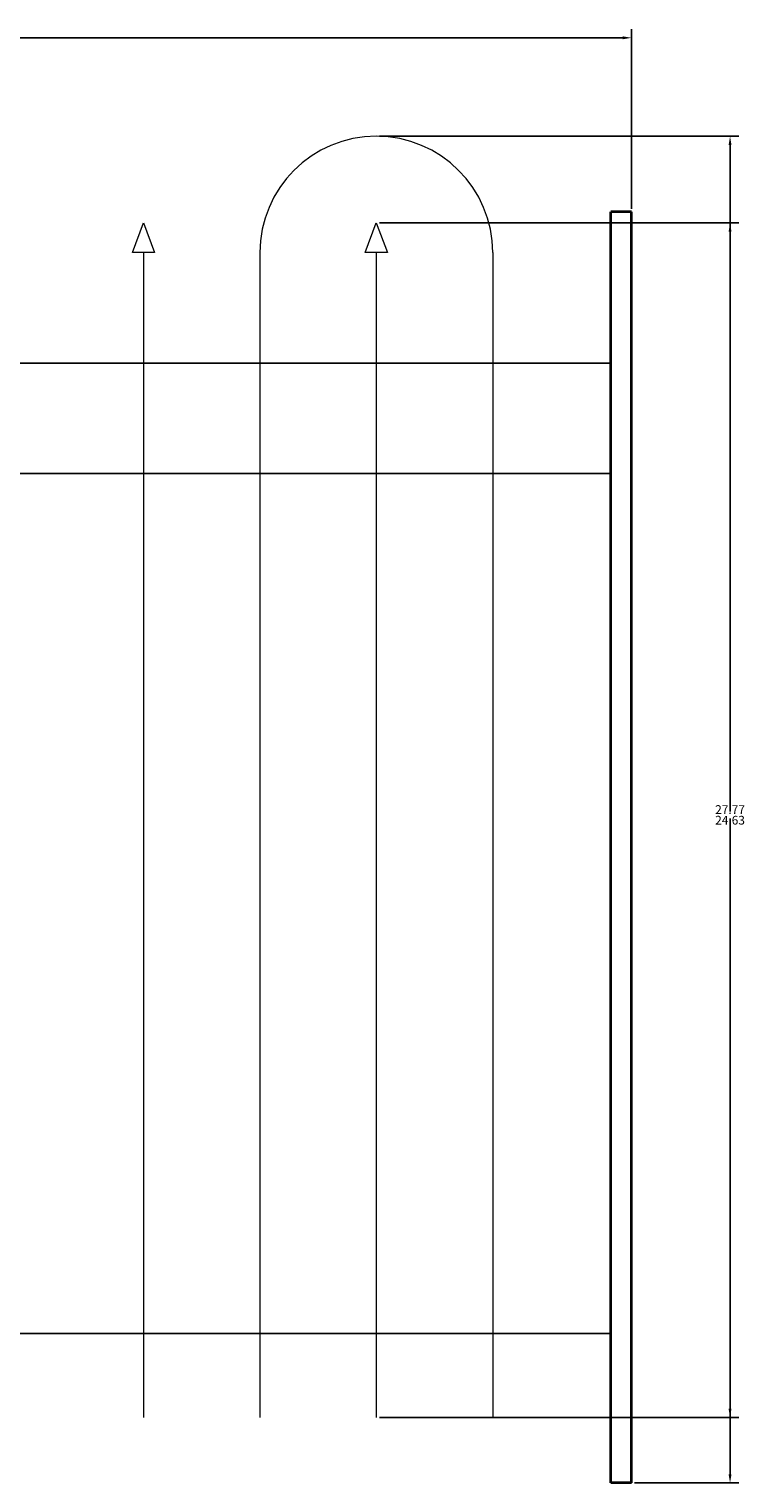
# Model space of a CAD drawing. Units: inches. Extents: x 756 to 915, y 488 to 695.
# Tile 14 of 25: x 844 to 859, y 594 to 624. Entities that reach past the tile are written whole.
import ezdxf

# ---------------------------------------------------------------- set-up
doc = ezdxf.new("R2010")
doc.units = ezdxf.units.IN
doc.header["$MEASUREMENT"] = 0
for name, color, linetype, lineweight in [('L-FENC-PCKT', 7, 'Continuous', 18), ('L-FENC-POST', 7, 'Continuous', 35), ('L-FENC-RAIL', 7, 'Continuous', 25), ('M-DIMS', 2, 'Continuous', 18)]:
    doc.layers.add(name, color=color, linetype=linetype, lineweight=lineweight)
doc.styles.get("Standard").update_dxf_attribs({"font": 'arial.ttf'})
doc.dimstyles.get("Standard").update_dxf_attribs({"dimtxt": 0.18, "dimasz": 0.18, "dimexe": 0.18, "dimexo": 0.0625, "dimgap": 0.09, "dimtad": 0, "dimtih": 1, "dimtoh": 1, "dimdec": 0, "dimzin": 0, "dimdsep": 46, "dimlunit": 3, "dimtxsty": 'Standard', "dimcen": 0.09, "dimadec": 0, "dimazin": 0, "dimtfac": 1, "dimtdec": 0, "dimtofl": 0, "dimtmove": 0, "dimatfit": 3, "dimfxl": 1, "dimtolj": 1, "dimtzin": 0, "dimarcsym": 0})

# ---------------------------------------------------------------- blocks, each defined once
blk = doc.blocks.new('FENCE-POST-RIGHT')
for p, q in [((0, 26.207), (0, 0)), ((0, 26.207), (0.427, 26.207)), ((0.427, 26.207), (0.427, 0)), ((0, 0), (0.427, 0))]:
    blk.add_line(p, q)
blk = doc.blocks.new('PICKET-ROUND-ARCH')
for p, q in [((0, 24.019), (0, 0)), ((4.8, 24.019), (4.8, 0))]:
    blk.add_line(p, q)
blk.add_arc((2.4, 24.019), 2.4, 0, 180)
blk = doc.blocks.new('PICKET-SPEAR-ARCH-INFILL')
blk.add_line((0.227, 24.019), (0.227, 0))
blk.add_lwpolyline([(0.227, 24.019), (0, 24.019), (0.227, 24.631), (0.455, 24.019)], close=True)
blk = doc.blocks.new('*D53')
at = {"layer": 'Defpoints', "color": 0, "transparency": 16777216}
for p in [(856.791, 623.683), (817.332, 620.092), (856.791, 620.092)]:
    blk.add_point(p, dxfattribs=at)
at = {"layer": 'M-DIMS', "color": 0, "lineweight": -2, "transparency": 16777216}
for p, q in [((817.332, 620.154), (817.332, 623.863)), ((856.791, 620.154), (856.791, 623.863)), ((817.512, 623.683), (836.668, 623.683)), ((856.611, 623.683), (837.455, 623.683))]:
    blk.add_line(p, q, dxfattribs=at)
at = {"layer": 'M-DIMS', "color": 0, "transparency": 16777216}
for points in [[(817.512, 623.713), (817.512, 623.653), (817.332, 623.683)], [(856.611, 623.713), (856.611, 623.653), (856.791, 623.683)]]:
    blk.add_solid(points, dxfattribs=at)
at = {"layer": 'M-DIMS', "color": 0, "transparency": 16777216, "insert": (837.062, 623.683), "char_height": 0.18, "attachment_point": 5}
blk.add_mtext('\\A1;39.46', dxfattribs=at)
blk = doc.blocks.new('*D54')
at = {"layer": 'Defpoints', "color": 0, "transparency": 16777216}
for p in [(851.53, 621.653), (858.821, 621.653), (856.791, 593.885)]:
    blk.add_point(p, dxfattribs=at)
at = {"layer": 'M-DIMS', "color": 0, "lineweight": -2, "transparency": 16777216}
for p, q in [((851.593, 621.653), (859.001, 621.653)), ((858.821, 621.473), (858.821, 607.949)), ((858.821, 594.065), (858.821, 607.588)), ((856.853, 593.885), (859.001, 593.885))]:
    blk.add_line(p, q, dxfattribs=at)
at = {"layer": 'M-DIMS', "color": 0, "transparency": 16777216}
for points in [[(858.791, 621.473), (858.851, 621.473), (858.821, 621.653)], [(858.791, 594.065), (858.851, 594.065), (858.821, 593.885)]]:
    blk.add_solid(points, dxfattribs=at)
at = {"layer": 'M-DIMS', "color": 0, "transparency": 16777216, "insert": (858.821, 607.769), "char_height": 0.18, "attachment_point": 5}
blk.add_mtext('\\A1;27.77', dxfattribs=at)
blk = doc.blocks.new('*D56')
at = {"layer": 'Defpoints', "color": 0, "transparency": 16777216}
for p in [(851.53, 619.865), (858.821, 619.865), (851.53, 595.234)]:
    blk.add_point(p, dxfattribs=at)
at = {"layer": 'M-DIMS', "color": 0, "lineweight": -2, "transparency": 16777216}
for p, q in [((851.593, 619.865), (859.001, 619.865)), ((858.821, 619.685), (858.821, 607.732)), ((858.821, 595.414), (858.821, 607.368)), ((851.593, 595.234), (859.001, 595.234))]:
    blk.add_line(p, q, dxfattribs=at)
at = {"layer": 'M-DIMS', "color": 0, "transparency": 16777216}
for points in [[(858.791, 619.685), (858.851, 619.685), (858.821, 619.865)], [(858.791, 595.414), (858.851, 595.414), (858.821, 595.234)]]:
    blk.add_solid(points, dxfattribs=at)
at = {"layer": 'M-DIMS', "color": 0, "transparency": 16777216, "insert": (858.821, 607.55), "char_height": 0.18, "attachment_point": 5}
blk.add_mtext('\\A1;24.63', dxfattribs=at)

msp = doc.modelspace()

# ---------------------------------------------------------------- linework, layer by layer
at = {"layer": 'L-FENC-RAIL'}
for p, q in [((817.7591, 616.9765), (856.3639, 616.9765)), ((817.7591, 614.7001), (856.3639, 614.7001)), ((817.7591, 596.9663), (856.3639, 596.9663))]:
    msp.add_line(p, q, dxfattribs=at)

# ---------------------------------------------------------------- block references
at = {"layer": 'L-FENC-PCKT'}
for name, p in [('PICKET-ROUND-ARCH', (849.13, 595.234)), ('PICKET-SPEAR-ARCH-INFILL', (846.5032, 595.234)), ('PICKET-SPEAR-ARCH-INFILL', (851.303, 595.234))]:
    msp.add_blockref(name, p, dxfattribs=at)
at = {"layer": 'L-FENC-POST', "rotation": 180}
msp.add_blockref('FENCE-POST-RIGHT', (856.7907, 620.0916), dxfattribs=at)

# ---------------------------------------------------------------- dimensions: what is measured, and where the dimension line sits
at = {"layer": 'M-DIMS'}
dim = msp.add_linear_dim(base=(856.7906, 623.6829), p1=(817.3324, 620.0915), p2=(856.7906, 620.0915), dimstyle='Standard', override={"dimdec": 2, "dimlfac": 1, "dimrnd": 0, "dimzin": 0, "dimdsep": 46, "dimlunit": 2}, dxfattribs=at)
dim.commit()
dim.dimension.update_dxf_attribs({"geometry": '*D53', "text_midpoint": (837.0615, 623.6829)})
for base, p1, p2, picture, middle in [((858.8206, 621.6529), (856.7906, 593.8847), (851.5304, 621.6529), '*D54', (858.8206, 607.7688)), ((858.8206, 619.8648), (851.5304, 595.2343), (851.5304, 619.8648), '*D56', (858.8206, 607.5496))]:
    dim = msp.add_linear_dim(base=base, p1=p1, p2=p2, angle=90, dimstyle='Standard', override={"dimdec": 2, "dimlfac": 1, "dimrnd": 0, "dimzin": 0, "dimdsep": 46, "dimlunit": 2}, dxfattribs=at)
    dim.commit()
    dim.dimension.update_dxf_attribs({"geometry": picture, "text_midpoint": middle})

doc.saveas('drawing.dxf')
